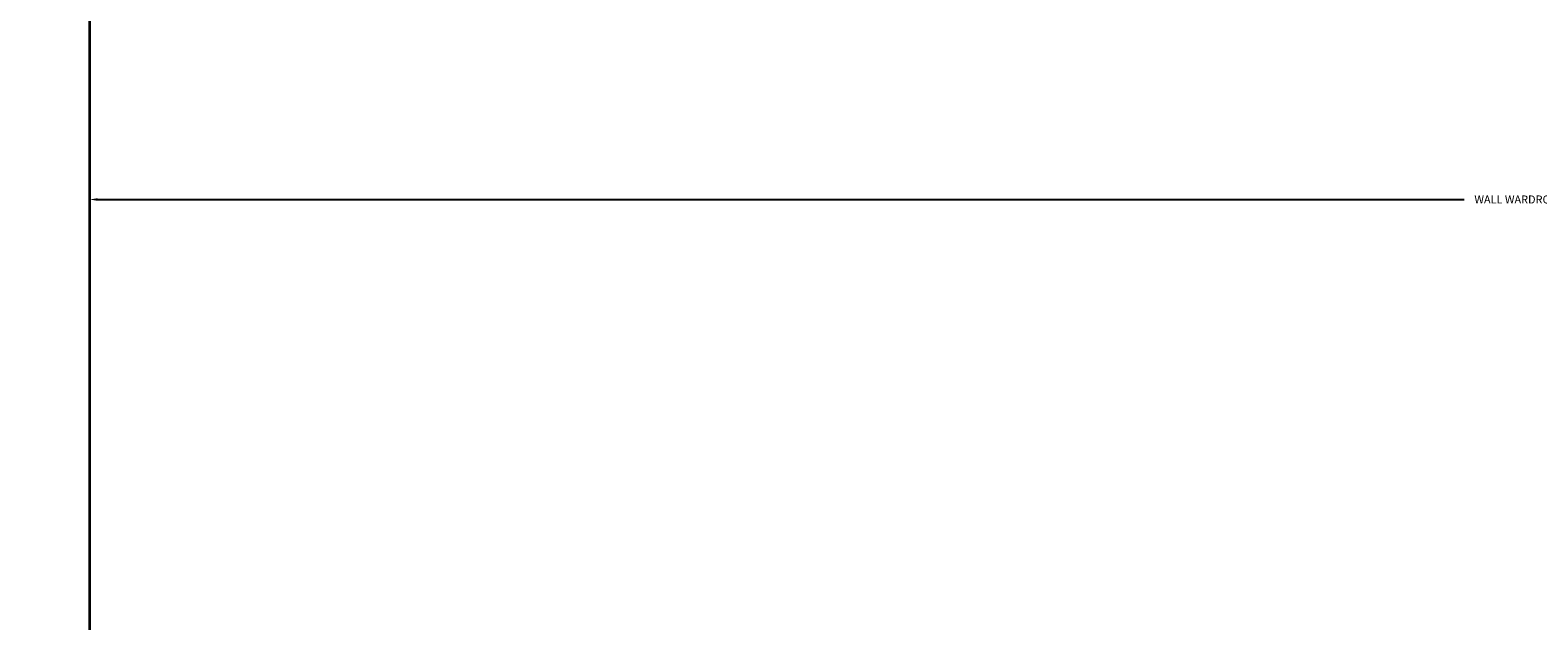
# Model space of a CAD drawing. Units: millimetres. Extents: x 27017497 to 27018854, y 7058029 to 7059154.
# Tile 39 of 91: x 27017621 to 27017655, y 7058459 to 7058472. Entities that reach past the tile are written whole.
import ezdxf

# ---------------------------------------------------------------- set-up
doc = ezdxf.new("R2010")
doc.units = ezdxf.units.MM
doc.layers.add('A-ANNO-DIMS', color=2, linetype='Continuous', lineweight=18)
doc.layers.add('A-WALL', color=7, linetype='Continuous', lineweight=35)
doc.styles.get("Standard").update_dxf_attribs({"font": 'arial.ttf'})
doc.dimstyles.get("Standard").update_dxf_attribs({"dimtxt": 0.18, "dimasz": 0.18, "dimexe": 0.18, "dimexo": 0.0625, "dimgap": 0.09, "dimtad": 0, "dimtih": 1, "dimtoh": 1, "dimdec": 4, "dimzin": 0, "dimdsep": 46, "dimtxsty": 'Standard', "dimcen": 0.09, "dimadec": 0, "dimazin": 0, "dimtfac": 1, "dimtdec": 4, "dimtofl": 0, "dimtmove": 0, "dimatfit": 3, "dimfxl": 1, "dimtolj": 1, "dimtzin": 0, "dimarcsym": 0})

# ---------------------------------------------------------------- blocks, each defined once
blk = doc.blocks.new('*D45')
at = {"layer": 'A-ANNO-DIMS', "color": 0, "lineweight": -2, "transparency": 16777216}
for p, q in [((27017622.665, 7058458.704), (27017622.665, 7058468.604)), ((27017687.877, 7058458.704), (27017687.877, 7058468.604)), ((27017622.845, 7058468.424), (27017653.586, 7058468.424)), ((27017687.697, 7058468.424), (27017656.955, 7058468.424))]:
    blk.add_line(p, q, dxfattribs=at)
at = {"layer": 'A-ANNO-DIMS', "color": 0, "transparency": 16777216}
for points in [[(27017622.845, 7058468.454), (27017622.845, 7058468.394), (27017622.665, 7058468.424)], [(27017687.697, 7058468.454), (27017687.697, 7058468.394), (27017687.877, 7058468.424)]]:
    blk.add_solid(points, dxfattribs=at)
at = {"layer": 'Defpoints', "color": 0, "transparency": 16777216}
for p in [(27017687.877, 7058468.424), (27017622.665, 7058458.642), (27017687.877, 7058458.642)]:
    blk.add_point(p, dxfattribs=at)
at = {"layer": 'A-ANNO-DIMS', "color": 0, "transparency": 16777216, "insert": (27017655.271, 7058468.424), "char_height": 0.18, "attachment_point": 5}
blk.add_mtext('\\A1;WALL WARDROBE 65 TYP.', dxfattribs=at)
blk = doc.blocks.new('*D48')
at = {"layer": 'A-ANNO-DIMS', "color": 0, "lineweight": -2, "transparency": 16777216}
for p, q in [((27018463.498, 7058622.912), (27017497.536, 7058622.912)), ((27017497.716, 7058622.732), (27017497.716, 7058357.753)), ((27017497.716, 7058092.41), (27017497.716, 7058357.389)), ((27018555.129, 7058092.23), (27017497.536, 7058092.23))]:
    blk.add_line(p, q, dxfattribs=at)
at = {"layer": 'A-ANNO-DIMS', "color": 0, "transparency": 16777216}
for points in [[(27017497.686, 7058622.732), (27017497.746, 7058622.732), (27017497.716, 7058622.912)], [(27017497.686, 7058092.41), (27017497.746, 7058092.41), (27017497.716, 7058092.23)]]:
    blk.add_solid(points, dxfattribs=at)
at = {"layer": 'Defpoints', "color": 0, "transparency": 16777216}
for p in [(27018463.561, 7058622.912), (27017497.716, 7058092.23), (27018555.192, 7058092.23)]:
    blk.add_point(p, dxfattribs=at)
at = {"layer": 'A-ANNO-DIMS', "color": 0, "transparency": 16777216, "insert": (27017497.716, 7058357.571), "char_height": 0.18, "attachment_point": 5}
blk.add_mtext('\\A1;530.7', dxfattribs=at)

msp = doc.modelspace()

# ---------------------------------------------------------------- linework, layer by layer
at = {"layer": 'A-WALL'}
msp.add_line((27017622.666, 7058580.912), (27017622.666, 7058436.912), dxfattribs=at)

# ---------------------------------------------------------------- dimensions: what is measured, and where the dimension line sits
at = {"layer": 'A-ANNO-DIMS'}
dim = msp.add_linear_dim(base=(27017497.716, 7058092.23), p1=(27018463.561, 7058622.912), p2=(27018555.192, 7058092.23), angle=90, dimstyle='Standard', override={"dimdec": 1, "dimlfac": 1, "dimrnd": 0, "dimzin": 0, "dimdsep": 46, "dimlunit": 2}, dxfattribs=at)
dim.commit()
dim.dimension.update_dxf_attribs({"geometry": '*D48', "text_midpoint": (27017497.716, 7058357.571)})
dim = msp.add_linear_dim(base=(27017687.877, 7058468.424), p1=(27017622.665, 7058458.642), p2=(27017687.877, 7058458.642), text='WALL WARDROBE <> TYP.', dimstyle='Standard', override={"dimdec": 0, "dimlfac": 1, "dimrnd": 0, "dimzin": 0, "dimdsep": 46, "dimlunit": 2}, dxfattribs=at)
dim.commit()
dim.dimension.update_dxf_attribs({"geometry": '*D45', "text_midpoint": (27017655.271, 7058468.424)})

doc.saveas('drawing.dxf')
